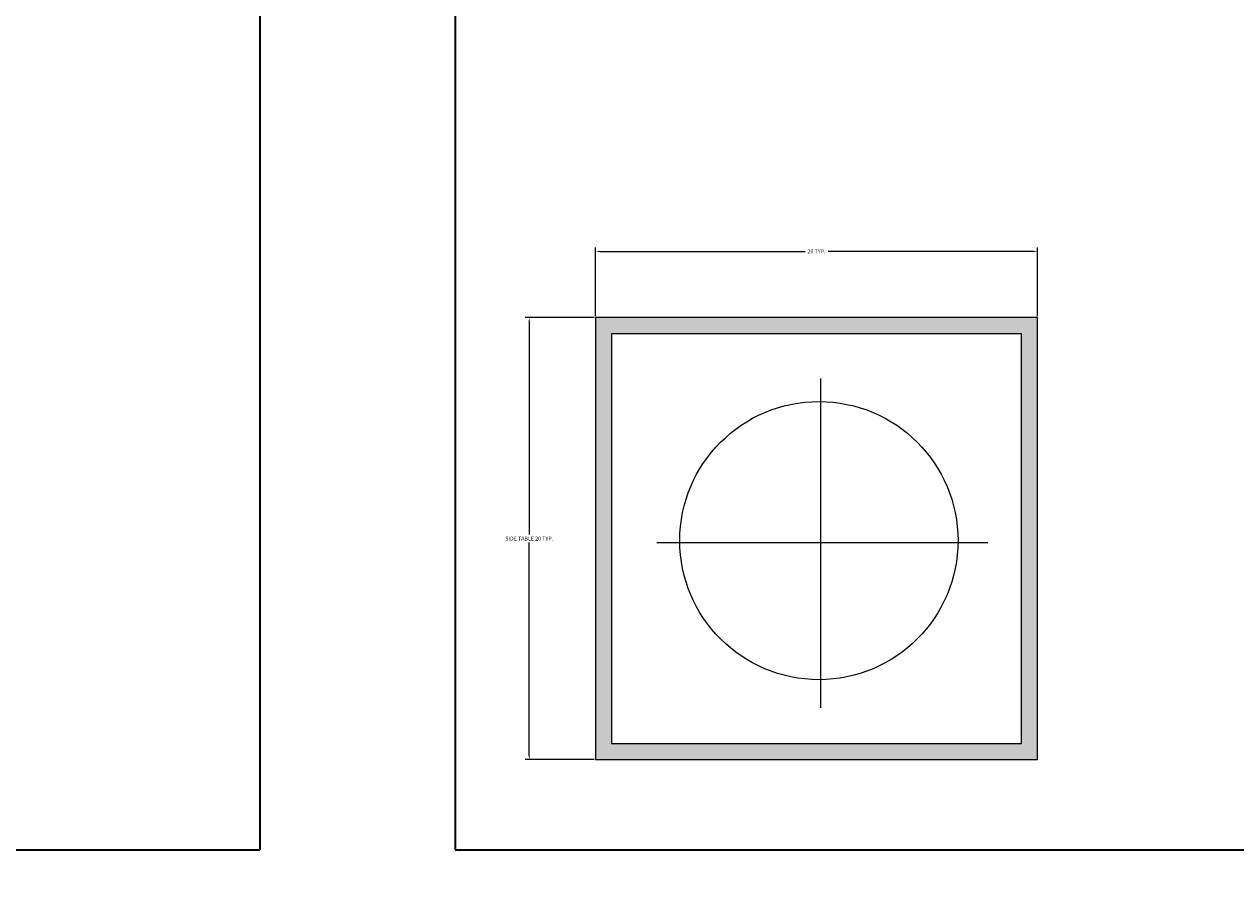
# Model space of a CAD drawing. Units: millimetres. Extents: x 27017497 to 27018854, y 7058029 to 7059154.
# Tile 32 of 91: x 27017621 to 27017677, y 7058297 to 7058337. Entities that reach past the tile are written whole.
import ezdxf

# ---------------------------------------------------------------- set-up
doc = ezdxf.new("R2010")
doc.units = ezdxf.units.MM
for name, color, linetype, lineweight in [('A-ANNO-DIMS', 2, 'Continuous', 18), ('A-FURN', 8, 'Continuous', 18), ('A-WALL', 7, 'Continuous', 35)]:
    doc.layers.add(name, color=color, linetype=linetype, lineweight=lineweight)
doc.layers.add('A-FURN-PATT', color=177, linetype='Continuous', lineweight=13, true_color=0x293189)
doc.styles.get("Standard").update_dxf_attribs({"font": 'arial.ttf'})
doc.dimstyles.get("Standard").update_dxf_attribs({"dimtxt": 0.18, "dimasz": 0.18, "dimexe": 0.18, "dimexo": 0.0625, "dimgap": 0.09, "dimtad": 0, "dimtih": 1, "dimtoh": 1, "dimdec": 4, "dimzin": 0, "dimdsep": 46, "dimtxsty": 'Standard', "dimcen": 0.09, "dimadec": 0, "dimazin": 0, "dimtfac": 1, "dimtdec": 4, "dimtofl": 0, "dimtmove": 0, "dimatfit": 3, "dimfxl": 1, "dimtolj": 1, "dimtzin": 0, "dimarcsym": 0})

# ---------------------------------------------------------------- blocks, each defined once
blk = doc.blocks.new('TABLE-END-LIVING')
for p, q in [((20.343, 20.343), (0, 20.343)), ((0, 20.343), (0, 0)), ((20.343, 0), (20.343, 20.343)), ((19.604, 19.604), (0.74, 19.604)), ((0.74, 19.604), (0.74, 0.74)), ((19.604, 0.74), (19.604, 19.604)), ((10.364, 2.372), (10.364, 17.538)), ((2.825, 9.996), (18.064, 9.996)), ((0.74, 0.74), (19.604, 0.74)), ((0, 0), (20.343, 0))]:
    blk.add_line(p, q)
blk.add_circle((10.282, 10.077), 6.403)
blk = doc.blocks.new('*D41')
at = {"layer": 'A-ANNO-DIMS', "color": 0, "lineweight": -2, "transparency": 16777216}
for p, q in [((27017647.561, 7058323.419), (27017644.392, 7058323.419)), ((27017644.572, 7058323.239), (27017644.572, 7058313.431)), ((27017644.572, 7058303.256), (27017644.572, 7058313.065)), ((27017647.561, 7058303.076), (27017644.392, 7058303.076))]:
    blk.add_line(p, q, dxfattribs=at)
at = {"layer": 'A-ANNO-DIMS', "color": 0, "transparency": 16777216}
for points in [[(27017644.542, 7058323.239), (27017644.602, 7058323.239), (27017644.572, 7058323.419)], [(27017644.542, 7058303.256), (27017644.602, 7058303.256), (27017644.572, 7058303.076)]]:
    blk.add_solid(points, dxfattribs=at)
at = {"layer": 'Defpoints', "color": 0, "transparency": 16777216}
for p in [(27017644.572, 7058323.419), (27017647.623, 7058323.419), (27017647.623, 7058303.076)]:
    blk.add_point(p, dxfattribs=at)
at = {"layer": 'A-ANNO-DIMS', "color": 0, "transparency": 16777216, "insert": (27017644.572, 7058313.248), "char_height": 0.18, "attachment_point": 5}
blk.add_mtext('\\A1;SIDE TABLE 20 TYP.', dxfattribs=at)
blk = doc.blocks.new('*D42')
at = {"layer": 'A-ANNO-DIMS', "color": 0, "lineweight": -2, "transparency": 16777216}
for p, q in [((27017647.623, 7058323.482), (27017647.623, 7058326.651)), ((27017667.966, 7058323.482), (27017667.966, 7058326.651)), ((27017647.803, 7058326.471), (27017657.265, 7058326.471)), ((27017667.786, 7058326.471), (27017658.324, 7058326.471))]:
    blk.add_line(p, q, dxfattribs=at)
at = {"layer": 'A-ANNO-DIMS', "color": 0, "transparency": 16777216}
for points in [[(27017647.803, 7058326.501), (27017647.803, 7058326.441), (27017647.623, 7058326.471)], [(27017667.786, 7058326.501), (27017667.786, 7058326.441), (27017667.966, 7058326.471)]]:
    blk.add_solid(points, dxfattribs=at)
at = {"layer": 'Defpoints', "color": 0, "transparency": 16777216}
for p in [(27017667.966, 7058326.471), (27017647.623, 7058323.419), (27017667.966, 7058323.419)]:
    blk.add_point(p, dxfattribs=at)
at = {"layer": 'A-ANNO-DIMS', "color": 0, "transparency": 16777216, "insert": (27017657.795, 7058326.471), "char_height": 0.18, "attachment_point": 5}
blk.add_mtext('\\A1;20 TYP.', dxfattribs=at)
blk = doc.blocks.new('*D48')
at = {"layer": 'A-ANNO-DIMS', "color": 0, "lineweight": -2, "transparency": 16777216}
for p, q in [((27018463.498, 7058622.912), (27017497.536, 7058622.912)), ((27017497.716, 7058622.732), (27017497.716, 7058357.753)), ((27017497.716, 7058092.41), (27017497.716, 7058357.389)), ((27018555.129, 7058092.23), (27017497.536, 7058092.23))]:
    blk.add_line(p, q, dxfattribs=at)
at = {"layer": 'A-ANNO-DIMS', "color": 0, "transparency": 16777216}
for points in [[(27017497.686, 7058622.732), (27017497.746, 7058622.732), (27017497.716, 7058622.912)], [(27017497.686, 7058092.41), (27017497.746, 7058092.41), (27017497.716, 7058092.23)]]:
    blk.add_solid(points, dxfattribs=at)
at = {"layer": 'Defpoints', "color": 0, "transparency": 16777216}
for p in [(27018463.561, 7058622.912), (27017497.716, 7058092.23), (27018555.192, 7058092.23)]:
    blk.add_point(p, dxfattribs=at)
at = {"layer": 'A-ANNO-DIMS', "color": 0, "transparency": 16777216, "insert": (27017497.716, 7058357.571), "char_height": 0.18, "attachment_point": 5}
blk.add_mtext('\\A1;530.7', dxfattribs=at)

msp = doc.modelspace()

# ---------------------------------------------------------------- hatches: boundary and pattern name
at = {"layer": 'A-FURN-PATT'}
h = msp.add_hatch(color=256, dxfattribs=at)
h.dxf.hatch_style = 1
h.paths.add_polyline_path([(27017667.966, 7058323.419), (27017647.623, 7058323.419), (27017647.623, 7058303.076), (27017667.966, 7058303.076)])
h.paths.add_polyline_path([(27017667.227, 7058322.68), (27017667.227, 7058303.816), (27017648.363, 7058303.816), (27017648.363, 7058322.68)], flags=16)
h.paths.add_polyline_path([(27017664.309, 7058313.153, -1), (27017651.502, 7058313.153, -1)], flags=0)

# ---------------------------------------------------------------- linework, layer by layer
at = {"layer": 'A-WALL'}
for p, q in [((27017632.166, 7058432.412), (27017632.166, 7058298.912)), ((27017641.166, 7058432.412), (27017641.166, 7058298.912)), ((27017565.666, 7058298.912), (27017632.166, 7058298.912)), ((27017641.166, 7058298.912), (27017743.666, 7058298.912))]:
    msp.add_line(p, q, dxfattribs=at)

# ---------------------------------------------------------------- block references
at = {"layer": 'A-FURN'}
msp.add_blockref('TABLE-END-LIVING', (27017647.623, 7058303.076), dxfattribs=at)

# ---------------------------------------------------------------- dimensions: what is measured, and where the dimension line sits
at = {"layer": 'A-ANNO-DIMS'}
dim = msp.add_linear_dim(base=(27017497.716, 7058092.23), p1=(27018463.561, 7058622.912), p2=(27018555.192, 7058092.23), angle=90, dimstyle='Standard', override={"dimdec": 1, "dimlfac": 1, "dimrnd": 0, "dimzin": 0, "dimdsep": 46, "dimlunit": 2}, dxfattribs=at)
dim.commit()
dim.dimension.update_dxf_attribs({"geometry": '*D48', "text_midpoint": (27017497.716, 7058357.571)})
dim = msp.add_linear_dim(base=(27017667.966, 7058326.471), p1=(27017647.623, 7058323.419), p2=(27017667.966, 7058323.419), text='<> TYP.', dimstyle='Standard', override={"dimdec": 0, "dimlfac": 1, "dimrnd": 0, "dimzin": 0, "dimdsep": 46, "dimlunit": 2}, dxfattribs=at)
dim.commit()
dim.dimension.update_dxf_attribs({"geometry": '*D42', "text_midpoint": (27017657.795, 7058326.471)})
dim = msp.add_linear_dim(base=(27017644.572, 7058323.419), p1=(27017647.623, 7058303.076), p2=(27017647.623, 7058323.419), angle=90, text='SIDE TABLE <> TYP.', dimstyle='Standard', override={"dimdec": 0, "dimlfac": 1, "dimrnd": 0, "dimzin": 0, "dimdsep": 46, "dimlunit": 2}, dxfattribs=at)
dim.commit()
dim.dimension.update_dxf_attribs({"geometry": '*D41', "text_midpoint": (27017644.572, 7058313.248)})

doc.saveas('drawing.dxf')
